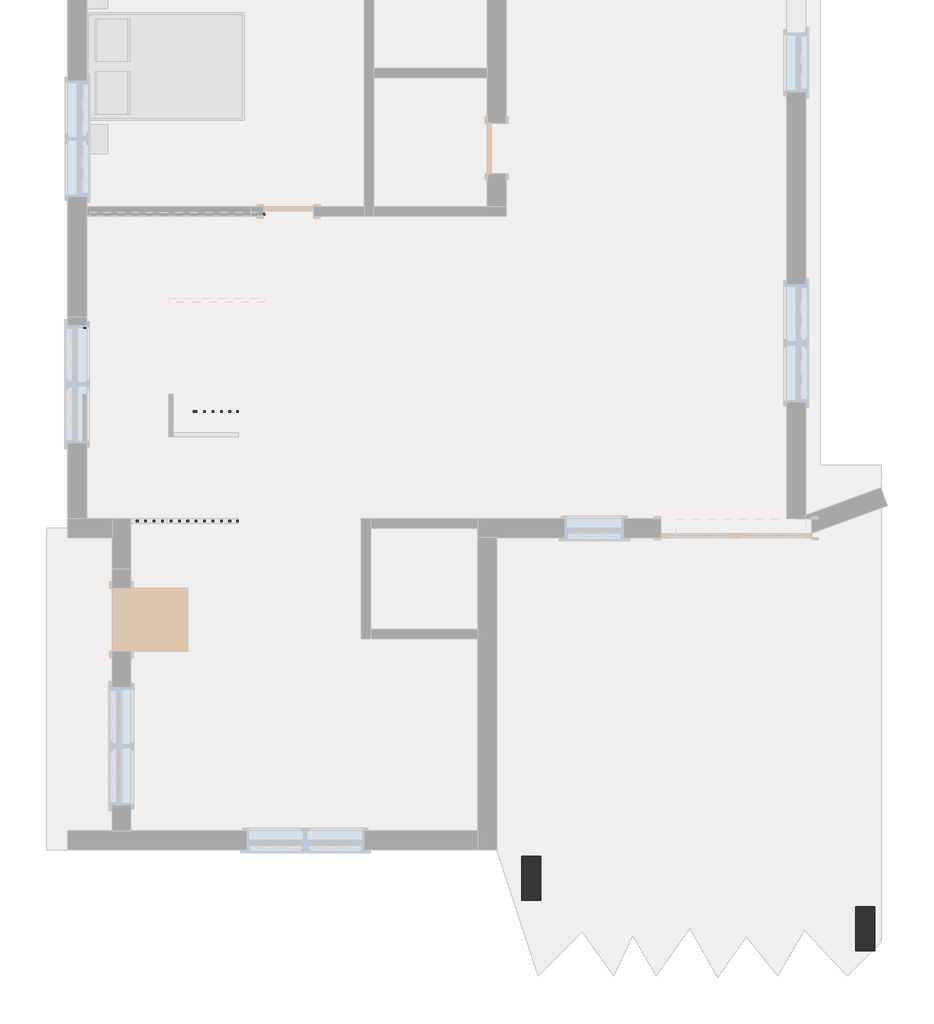
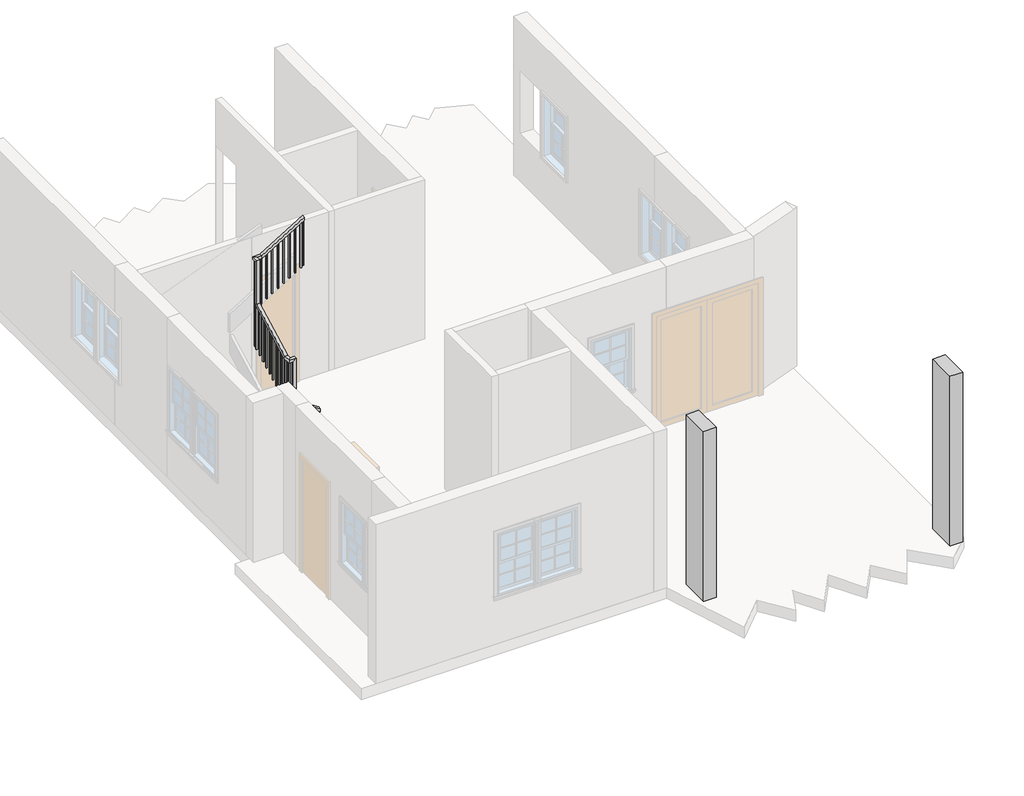
# One storey, part 2 of 3: 2 columns, 2 railings.
"""IFC4 building model written with IfcOpenShell, lengths in millimetres."""

from ifc_helpers import new_model, si_unit, frame, origin, place, context, project, spatial, polyline, outline, extrude, faceted_brep, transform, mapped, element, save
from components import column_b42c64cd

model = new_model("IFC4")

# Units and contexts
model_context = context("Model", 3, world=origin())
ifc_project = project(units=[si_unit("LENGTHUNIT", "METRE", prefix="MILLI")], contexts=[model_context])

# Site, building, storey
site = spatial("IfcSite", under=ifc_project)
building = spatial("IfcBuilding", under=site)
storey = spatial("IfcBuildingStorey", under=building, Elevation=3200.4)

# Columns
placement = place(None, origin())
column_shape = column_b42c64cd(model_context)
element("IfcColumn", 1, ObjectType="Rectangular Column : x9\"", at=placement, inside=storey, context=model_context, shape_type="MappedRepresentation", body=[
    mapped(column_shape, transform((-16875.4750314, 319.9223646, 0.0), x_axis=(1.0, 0.0, 0.0), y_axis=(0.0, 1.0, 0.0), z_axis=(0.0, 0.0, 1.0))),
])
element("IfcColumn", 2, ObjectType="Rectangular Column : x9\"", at=placement, inside=storey, context=model_context, shape_type="MappedRepresentation", body=[
    mapped(column_shape, transform((-12836.8750314, -289.6776354, 0.0), x_axis=(1.0, 0.0, 0.0), y_axis=(0.0, 1.0, 0.0), z_axis=(0.0, 0.0, 1.0))),
])

# Railings
element("IfcRailing", 3, ObjectType="Handrail - Rectangular", at=placement, inside=storey, context=model_context, shape_type="SolidModel", body=[
    faceted_brep([(-20418.7750314, 5933.3223646, 4470.4), (-20418.7750314, 5933.3223646, 4410.186276), (-20418.7750314, 5984.1223646, 4410.186276), (-20418.7750314, 5984.1223646, 4470.4), (-20850.5750314, 5933.3223646, 4745.1818182), (-20901.3750314, 5933.3223646, 4717.2953669), (-20901.3750314, 5984.1223646, 4717.2953669), (-20850.5750314, 5984.1223646, 4745.1818182), (-20850.5750314, 5933.3223646, 5574.9151515), (-20901.3750314, 5933.3223646, 5524.1151515), (-20901.3750314, 5984.1223646, 5524.1151515), (-20850.5750314, 5984.1223646, 5574.9151515), (-20977.5750314, 5933.3223646, 5574.9151515), (-20977.5750314, 5933.3223646, 5524.1151515), (-20926.7750314, 5984.1223646, 5524.1151515), (-20926.7750314, 5984.1223646, 5574.9151515), (-20977.5750314, 6060.3223646, 5574.9151515), (-20977.5750314, 6072.9586335, 5524.1151515), (-20926.7750314, 6072.9586335, 5524.1151515), (-20926.7750314, 6060.3223646, 5574.9151515), (-20977.5750314, 6923.9223646, 6032.8848485), (-20977.5750314, 6974.7223646, 6002.3231907), (-20926.7750314, 6974.7223646, 6002.3231907), (-20926.7750314, 6923.9223646, 6032.8848485), (-20088.5750314, 7050.9223646, 7315.2), (-20088.5750314, 7000.1223646, 7315.2), (-20088.5750314, 7000.1223646, 7255.7290495), (-20088.5750314, 7050.9223646, 7255.7290495), (-20836.3298984, 7050.9223646, 6800.573913), (-20850.5750314, 7050.9223646, 6851.373913), (-20836.3298984, 7000.1223646, 6800.573913), (-20850.5750314, 7000.1223646, 6851.373913), (-20977.5750314, 6923.9223646, 6851.373913), (-20977.5750314, 6974.7223646, 6800.573913), (-20926.7750314, 6974.7223646, 6800.573913), (-20926.7750314, 6923.9223646, 6851.373913), (-20977.5750314, 7050.9223646, 6851.373913), (-20977.5750314, 7050.9223646, 6800.573913), (-20926.7750314, 7000.1223646, 6800.573913), (-20926.7750314, 7000.1223646, 6851.373913)], [[[0, 1, 2, 3]], [[1, 0, 4, 5]], [[2, 1, 5, 6]], [[3, 2, 6, 7]], [[0, 3, 7, 4]], [[5, 4, 8, 9]], [[6, 5, 9, 10]], [[7, 6, 10, 11]], [[4, 7, 11, 8]], [[9, 8, 12, 13]], [[10, 9, 13, 14]], [[11, 10, 14, 15]], [[8, 11, 15, 12]], [[13, 12, 16, 17]], [[14, 13, 17, 18]], [[15, 14, 18, 19]], [[12, 15, 19, 16]], [[17, 16, 20, 21]], [[18, 17, 21, 22]], [[19, 18, 22, 23]], [[16, 19, 23, 20]], [[24, 25, 26, 27]], [[28, 29, 24, 27]], [[30, 28, 27, 26]], [[31, 30, 26, 25]], [[29, 31, 25, 24]], [[21, 20, 32, 33]], [[22, 21, 33, 34]], [[23, 22, 34, 35]], [[20, 23, 35, 32]], [[33, 32, 36, 37]], [[34, 33, 37, 38]], [[35, 34, 38, 39]], [[32, 35, 39, 36]], [[37, 36, 29, 28]], [[38, 37, 28, 30]], [[39, 38, 30, 31]], [[36, 39, 31, 29]]]),
    extrude(outline(polyline([(7230.6051365, -20129.8500314), (7219.0094843, -20148.9000314), (6369.8782609, -20148.9000314), (6369.8782609, -20129.8500314), (7230.6051365, -20129.8500314)])), frame((0.0, 7015.9973646, 0.0), z_axis=(0.0, 1.0, 0.0), x_axis=(0.0, 0.0, 1.0)), (0.0, 0.0, 1.0), 19.05),
    extrude(outline(polyline([(7168.7616582, -20231.4500314), (7157.166006, -20250.5000314), (6308.0347826, -20250.5000314), (6308.0347826, -20231.4500314), (7168.7616582, -20231.4500314)])), frame((0.0, 7015.9973646, 0.0), z_axis=(0.0, 1.0, 0.0), x_axis=(0.0, 0.0, 1.0)), (0.0, 0.0, 1.0), 19.05),
    extrude(outline(polyline([(7106.91818, -20333.0500314), (7095.3225278, -20352.1000314), (6246.1913043, -20352.1000314), (6246.1913043, -20333.0500314), (7106.91818, -20333.0500314)])), frame((0.0, 7015.9973646, 0.0), z_axis=(0.0, 1.0, 0.0), x_axis=(0.0, 0.0, 1.0)), (0.0, 0.0, 1.0), 19.05),
    extrude(outline(polyline([(7045.0747017, -20434.6500314), (7033.4790495, -20453.7000314), (6184.3478261, -20453.7000314), (6184.3478261, -20434.6500314), (7045.0747017, -20434.6500314)])), frame((0.0, 7015.9973646, 0.0), z_axis=(0.0, 1.0, 0.0), x_axis=(0.0, 0.0, 1.0)), (0.0, 0.0, 1.0), 19.05),
    extrude(outline(polyline([(6983.2312234, -20536.2500314), (6971.6355713, -20555.3000314), (6122.5043478, -20555.3000314), (6122.5043478, -20536.2500314), (6983.2312234, -20536.2500314)])), frame((0.0, 7015.9973646, 0.0), z_axis=(0.0, 1.0, 0.0), x_axis=(0.0, 0.0, 1.0)), (0.0, 0.0, 1.0), 19.05),
    extrude(outline(polyline([(6921.3877452, -20637.8500314), (6909.792093, -20656.9000314), (6060.6608696, -20656.9000314), (6060.6608696, -20637.8500314), (6921.3877452, -20637.8500314)])), frame((0.0, 7015.9973646, 0.0), z_axis=(0.0, 1.0, 0.0), x_axis=(0.0, 0.0, 1.0)), (0.0, 0.0, 1.0), 19.05),
    extrude(outline(polyline([(6859.5442669, -20739.4500314), (6847.9486147, -20758.5000314), (5998.8173913, -20758.5000314), (5998.8173913, -20739.4500314), (6859.5442669, -20739.4500314)])), frame((0.0, 7015.9973646, 0.0), z_axis=(0.0, 1.0, 0.0), x_axis=(0.0, 0.0, 1.0)), (0.0, 0.0, 1.0), 19.05),
    extrude(outline(polyline([(6797.7007887, -20841.0500314), (6786.1051365, -20860.1000314), (5936.973913, -20860.1000314), (5936.973913, -20841.0500314), (6797.7007887, -20841.0500314)])), frame((0.0, 7015.9973646, 0.0), z_axis=(0.0, 1.0, 0.0), x_axis=(0.0, 0.0, 1.0)), (0.0, 0.0, 1.0), 19.05),
    extrude(outline(polyline([(-20942.6500314, 6965.1973646), (-20961.7000314, 6965.1973646), (-20961.7000314, 6984.2473646), (-20942.6500314, 6984.2473646), (-20942.6500314, 6965.1973646)])), frame((0.0, 0.0, 5145.4242424), z_axis=(0.0, 0.0, 1.0), x_axis=(1.0, 0.0, 0.0)), (0.0, 0.0, 1.0), 1655.1496706),
    extrude(outline(polyline([(6863.5973646, 5943.3932665), (6882.6473646, 5953.4955392), (6882.6473646, 5091.5454545), (6863.5973646, 5091.5454545), (6863.5973646, 5943.3932665)])), frame((-20961.7000314, 0.0, 0.0), z_axis=(1.0, 0.0, 0.0), x_axis=(0.0, 1.0, 0.0)), (0.0, 0.0, 1.0), 19.05),
    extrude(outline(polyline([(6761.9973646, 5889.5144786), (6781.0473646, 5899.6167513), (6781.0473646, 5037.6666667), (6761.9973646, 5037.6666667), (6761.9973646, 5889.5144786)])), frame((-20961.7000314, 0.0, 0.0), z_axis=(1.0, 0.0, 0.0), x_axis=(0.0, 1.0, 0.0)), (0.0, 0.0, 1.0), 19.05),
    extrude(outline(polyline([(6660.3973646, 5835.6356907), (6679.4473646, 5845.7379635), (6679.4473646, 4983.7878788), (6660.3973646, 4983.7878788), (6660.3973646, 5835.6356907)])), frame((-20961.7000314, 0.0, 0.0), z_axis=(1.0, 0.0, 0.0), x_axis=(0.0, 1.0, 0.0)), (0.0, 0.0, 1.0), 19.05),
    extrude(outline(polyline([(6558.7973646, 5781.7569029), (6577.8473646, 5791.8591756), (6577.8473646, 4929.9090909), (6558.7973646, 4929.9090909), (6558.7973646, 5781.7569029)])), frame((-20961.7000314, 0.0, 0.0), z_axis=(1.0, 0.0, 0.0), x_axis=(0.0, 1.0, 0.0)), (0.0, 0.0, 1.0), 19.05),
    extrude(outline(polyline([(6457.1973646, 5727.878115), (6476.2473646, 5737.9803877), (6476.2473646, 4876.030303), (6457.1973646, 4876.030303), (6457.1973646, 5727.878115)])), frame((-20961.7000314, 0.0, 0.0), z_axis=(1.0, 0.0, 0.0), x_axis=(0.0, 1.0, 0.0)), (0.0, 0.0, 1.0), 19.05),
    extrude(outline(polyline([(6355.5973646, 5673.9993271), (6374.6473646, 5684.1015998), (6374.6473646, 4822.1515152), (6355.5973646, 4822.1515152), (6355.5973646, 5673.9993271)])), frame((-20961.7000314, 0.0, 0.0), z_axis=(1.0, 0.0, 0.0), x_axis=(0.0, 1.0, 0.0)), (0.0, 0.0, 1.0), 19.05),
    extrude(outline(polyline([(6253.9973646, 5620.1205392), (6273.0473646, 5630.2228119), (6273.0473646, 4768.2727273), (6253.9973646, 4768.2727273), (6253.9973646, 5620.1205392)])), frame((-20961.7000314, 0.0, 0.0), z_axis=(1.0, 0.0, 0.0), x_axis=(0.0, 1.0, 0.0)), (0.0, 0.0, 1.0), 19.05),
    extrude(outline(polyline([(6152.3973646, 5566.2417513), (6171.4473646, 5576.3440241), (6171.4473646, 4714.3939394), (6152.3973646, 4714.3939394), (6152.3973646, 5566.2417513)])), frame((-20961.7000314, 0.0, 0.0), z_axis=(1.0, 0.0, 0.0), x_axis=(0.0, 1.0, 0.0)), (0.0, 0.0, 1.0), 19.05),
    extrude(outline(polyline([(6050.7973646, 5512.3629635), (6069.8473646, 5522.4652362), (6069.8473646, 4660.5151515), (6050.7973646, 4660.5151515), (6050.7973646, 5512.3629635)])), frame((-20961.7000314, 0.0, 0.0), z_axis=(1.0, 0.0, 0.0), x_axis=(0.0, 1.0, 0.0)), (0.0, 0.0, 1.0), 19.05),
    extrude(outline(polyline([(-20917.2500314, 5968.2473646), (-20917.2500314, 5949.1973646), (-20936.3000314, 5949.1973646), (-20936.3000314, 5968.2473646), (-20917.2500314, 5968.2473646)])), frame((0.0, 0.0, 3879.2727273), z_axis=(0.0, 0.0, 1.0), x_axis=(1.0, 0.0, 0.0)), (0.0, 0.0, 1.0), 1644.8424242),
    extrude(outline(polyline([(4662.7430941, -20815.6500314), (4674.8658214, -20834.7000314), (3814.6181818, -20834.7000314), (3814.6181818, -20815.6500314), (4662.7430941, -20815.6500314)])), frame((0.0, 5949.1973646, 0.0), z_axis=(0.0, 1.0, 0.0), x_axis=(0.0, 0.0, 1.0)), (0.0, 0.0, 1.0), 19.05),
    extrude(outline(polyline([(4598.0885487, -20714.0500314), (4610.211276, -20733.1000314), (3749.9636364, -20733.1000314), (3749.9636364, -20714.0500314), (4598.0885487, -20714.0500314)])), frame((0.0, 5949.1973646, 0.0), z_axis=(0.0, 1.0, 0.0), x_axis=(0.0, 0.0, 1.0)), (0.0, 0.0, 1.0), 19.05),
    extrude(outline(polyline([(4533.4340032, -20612.4500314), (4545.5567305, -20631.5000314), (3685.3090909, -20631.5000314), (3685.3090909, -20612.4500314), (4533.4340032, -20612.4500314)])), frame((0.0, 5949.1973646, 0.0), z_axis=(0.0, 1.0, 0.0), x_axis=(0.0, 0.0, 1.0)), (0.0, 0.0, 1.0), 19.05),
    extrude(outline(polyline([(4468.7794578, -20510.8500314), (4480.9021851, -20529.9000314), (3620.6545455, -20529.9000314), (3620.6545455, -20510.8500314), (4468.7794578, -20510.8500314)])), frame((0.0, 5949.1973646, 0.0), z_axis=(0.0, 1.0, 0.0), x_axis=(0.0, 0.0, 1.0)), (0.0, 0.0, 1.0), 19.05),
    extrude(outline(polyline([(-20942.6500314, 7015.9973646), (-20961.7000314, 7015.9973646), (-20961.7000314, 7035.0473646), (-20942.6500314, 7035.0473646), (-20942.6500314, 7015.9973646)])), frame((0.0, 0.0, 5172.3636364), z_axis=(0.0, 0.0, 1.0), x_axis=(1.0, 0.0, 0.0)), (0.0, 0.0, 1.0), 1628.2102767),
    extrude(outline(polyline([(-20942.6500314, 5968.2473646), (-20942.6500314, 5949.1973646), (-20961.7000314, 5949.1973646), (-20961.7000314, 5968.2473646), (-20942.6500314, 5968.2473646)])), frame((0.0, 0.0, 3895.4363636), z_axis=(0.0, 0.0, 1.0), x_axis=(1.0, 0.0, 0.0)), (0.0, 0.0, 1.0), 1628.6787879),
    extrude(outline(polyline([(7255.7290495, -20088.5750314), (7244.1333973, -20107.6250314), (6395.0021739, -20107.6250314), (6395.0021739, -20088.5750314), (7255.7290495, -20088.5750314)])), frame((0.0, 7015.9973646, 0.0), z_axis=(0.0, 1.0, 0.0), x_axis=(0.0, 0.0, 1.0)), (0.0, 0.0, 1.0), 19.05),
    extrude(outline(polyline([(4410.186276, -20418.7750314), (4422.3090032, -20437.8250314), (3562.0613636, -20437.8250314), (3562.0613636, -20418.7750314), (4410.186276, -20418.7750314)])), frame((0.0, 5949.1973646, 0.0), z_axis=(0.0, 1.0, 0.0), x_axis=(0.0, 0.0, 1.0)), (0.0, 0.0, 1.0), 19.05),
])
element("IfcRailing", 4, ObjectType="Handrail - Rectangular", at=placement, inside=storey, context=model_context, shape_type="SolidModel", body=[
    faceted_brep([(-20418.7750314, 4612.5223646, 4470.4), (-20418.7750314, 4612.5223646, 4415.8938354), (-20418.7750314, 4663.3223646, 4415.8938354), (-20418.7750314, 4663.3223646, 4470.4), (-22171.3752061, 4612.5223646, 5151.9667346), (-22222.1752061, 4612.5223646, 5117.2161256), (-22222.1752061, 4663.3223646, 5117.2161256), (-22171.3752061, 4663.3223646, 5151.9667346), (-22171.3752061, 4612.5223646, 5181.600068), (-22222.1752061, 4612.5223646, 5130.800068), (-22222.1752061, 4663.3223646, 5130.800068), (-22171.3752061, 4663.3223646, 5181.600068), (-22298.3752061, 4612.5223646, 5181.600068), (-22298.3752061, 4612.5223646, 5130.800068), (-22247.5752061, 4663.3223646, 5130.800068), (-22247.5752061, 4663.3223646, 5181.600068), (-22298.3752061, 4739.5223646, 5181.600068), (-22298.3752061, 4739.5223646, 5130.800068), (-22247.5752061, 4739.5223646, 5130.800068), (-22247.5752061, 4739.5223646, 5181.600068), (-22298.3752061, 8371.7223646, 5181.600068), (-22298.3752061, 8371.7223646, 5130.800068), (-22247.5752061, 8320.9223646, 5130.800068), (-22247.5752061, 8320.9223646, 5181.600068), (-20088.5750314, 8371.7223646, 5181.600068), (-20088.5750314, 8320.9223646, 5181.600068), (-20088.5750314, 8320.9223646, 5130.800068), (-20088.5750314, 8371.7223646, 5130.800068)], [[[0, 1, 2, 3]], [[1, 0, 4, 5]], [[2, 1, 5, 6]], [[3, 2, 6, 7]], [[0, 3, 7, 4]], [[5, 4, 8, 9]], [[6, 5, 9, 10]], [[7, 6, 10, 11]], [[4, 7, 11, 8]], [[9, 8, 12, 13]], [[10, 9, 13, 14]], [[11, 10, 14, 15]], [[8, 11, 15, 12]], [[13, 12, 16, 17]], [[14, 13, 17, 18]], [[15, 14, 18, 19]], [[12, 15, 19, 16]], [[17, 16, 20, 21]], [[18, 17, 21, 22]], [[19, 18, 22, 23]], [[16, 19, 23, 20]], [[24, 25, 26, 27]], [[21, 20, 24, 27]], [[22, 21, 27, 26]], [[23, 22, 26, 25]], [[20, 23, 25, 24]]]),
    extrude(outline(polyline([(-20148.9002061, 8355.8473646), (-20129.8502061, 8355.8473646), (-20129.8502061, 8336.7973646), (-20148.9002061, 8336.7973646), (-20148.9002061, 8355.8473646)])), frame((0.0, 0.0, 4267.200068), z_axis=(0.0, 0.0, 1.0), x_axis=(1.0, 0.0, 0.0)), (0.0, 0.0, 1.0), 863.6),
    extrude(outline(polyline([(-20250.5002061, 8355.8473646), (-20231.4502061, 8355.8473646), (-20231.4502061, 8336.7973646), (-20250.5002061, 8336.7973646), (-20250.5002061, 8355.8473646)])), frame((0.0, 0.0, 4267.200068), z_axis=(0.0, 0.0, 1.0), x_axis=(1.0, 0.0, 0.0)), (0.0, 0.0, 1.0), 863.6),
    extrude(outline(polyline([(-20352.1002061, 8355.8473646), (-20333.0502061, 8355.8473646), (-20333.0502061, 8336.7973646), (-20352.1002061, 8336.7973646), (-20352.1002061, 8355.8473646)])), frame((0.0, 0.0, 4267.200068), z_axis=(0.0, 0.0, 1.0), x_axis=(1.0, 0.0, 0.0)), (0.0, 0.0, 1.0), 863.6),
    extrude(outline(polyline([(-20453.7002061, 8355.8473646), (-20434.6502061, 8355.8473646), (-20434.6502061, 8336.7973646), (-20453.7002061, 8336.7973646), (-20453.7002061, 8355.8473646)])), frame((0.0, 0.0, 4267.200068), z_axis=(0.0, 0.0, 1.0), x_axis=(1.0, 0.0, 0.0)), (0.0, 0.0, 1.0), 863.6),
    extrude(outline(polyline([(-20555.3002061, 8355.8473646), (-20536.2502061, 8355.8473646), (-20536.2502061, 8336.7973646), (-20555.3002061, 8336.7973646), (-20555.3002061, 8355.8473646)])), frame((0.0, 0.0, 4267.200068), z_axis=(0.0, 0.0, 1.0), x_axis=(1.0, 0.0, 0.0)), (0.0, 0.0, 1.0), 863.6),
    extrude(outline(polyline([(-20656.9002061, 8355.8473646), (-20637.8502061, 8355.8473646), (-20637.8502061, 8336.7973646), (-20656.9002061, 8336.7973646), (-20656.9002061, 8355.8473646)])), frame((0.0, 0.0, 4267.200068), z_axis=(0.0, 0.0, 1.0), x_axis=(1.0, 0.0, 0.0)), (0.0, 0.0, 1.0), 863.6),
    extrude(outline(polyline([(-20758.5002061, 8355.8473646), (-20739.4502061, 8355.8473646), (-20739.4502061, 8336.7973646), (-20758.5002061, 8336.7973646), (-20758.5002061, 8355.8473646)])), frame((0.0, 0.0, 4267.200068), z_axis=(0.0, 0.0, 1.0), x_axis=(1.0, 0.0, 0.0)), (0.0, 0.0, 1.0), 863.6),
    extrude(outline(polyline([(-20860.1002061, 8355.8473646), (-20841.0502061, 8355.8473646), (-20841.0502061, 8336.7973646), (-20860.1002061, 8336.7973646), (-20860.1002061, 8355.8473646)])), frame((0.0, 0.0, 4267.200068), z_axis=(0.0, 0.0, 1.0), x_axis=(1.0, 0.0, 0.0)), (0.0, 0.0, 1.0), 863.6),
    extrude(outline(polyline([(-20961.7002061, 8355.8473646), (-20942.6502061, 8355.8473646), (-20942.6502061, 8336.7973646), (-20961.7002061, 8336.7973646), (-20961.7002061, 8355.8473646)])), frame((0.0, 0.0, 4267.200068), z_axis=(0.0, 0.0, 1.0), x_axis=(1.0, 0.0, 0.0)), (0.0, 0.0, 1.0), 863.6),
    extrude(outline(polyline([(-21063.3002061, 8355.8473646), (-21044.2502061, 8355.8473646), (-21044.2502061, 8336.7973646), (-21063.3002061, 8336.7973646), (-21063.3002061, 8355.8473646)])), frame((0.0, 0.0, 4267.200068), z_axis=(0.0, 0.0, 1.0), x_axis=(1.0, 0.0, 0.0)), (0.0, 0.0, 1.0), 863.6),
    extrude(outline(polyline([(-21164.9002061, 8355.8473646), (-21145.8502061, 8355.8473646), (-21145.8502061, 8336.7973646), (-21164.9002061, 8336.7973646), (-21164.9002061, 8355.8473646)])), frame((0.0, 0.0, 4267.200068), z_axis=(0.0, 0.0, 1.0), x_axis=(1.0, 0.0, 0.0)), (0.0, 0.0, 1.0), 863.6),
    extrude(outline(polyline([(-21266.5002061, 8355.8473646), (-21247.4502061, 8355.8473646), (-21247.4502061, 8336.7973646), (-21266.5002061, 8336.7973646), (-21266.5002061, 8355.8473646)])), frame((0.0, 0.0, 4267.200068), z_axis=(0.0, 0.0, 1.0), x_axis=(1.0, 0.0, 0.0)), (0.0, 0.0, 1.0), 863.6),
    extrude(outline(polyline([(-21368.1002061, 8355.8473646), (-21349.0502061, 8355.8473646), (-21349.0502061, 8336.7973646), (-21368.1002061, 8336.7973646), (-21368.1002061, 8355.8473646)])), frame((0.0, 0.0, 4267.200068), z_axis=(0.0, 0.0, 1.0), x_axis=(1.0, 0.0, 0.0)), (0.0, 0.0, 1.0), 863.6),
    extrude(outline(polyline([(-21469.7002061, 8355.8473646), (-21450.6502061, 8355.8473646), (-21450.6502061, 8336.7973646), (-21469.7002061, 8336.7973646), (-21469.7002061, 8355.8473646)])), frame((0.0, 0.0, 4267.200068), z_axis=(0.0, 0.0, 1.0), x_axis=(1.0, 0.0, 0.0)), (0.0, 0.0, 1.0), 863.6),
    extrude(outline(polyline([(-21571.3002061, 8355.8473646), (-21552.2502061, 8355.8473646), (-21552.2502061, 8336.7973646), (-21571.3002061, 8336.7973646), (-21571.3002061, 8355.8473646)])), frame((0.0, 0.0, 4267.200068), z_axis=(0.0, 0.0, 1.0), x_axis=(1.0, 0.0, 0.0)), (0.0, 0.0, 1.0), 863.6),
    extrude(outline(polyline([(-21672.9002061, 8355.8473646), (-21653.8502061, 8355.8473646), (-21653.8502061, 8336.7973646), (-21672.9002061, 8336.7973646), (-21672.9002061, 8355.8473646)])), frame((0.0, 0.0, 4267.200068), z_axis=(0.0, 0.0, 1.0), x_axis=(1.0, 0.0, 0.0)), (0.0, 0.0, 1.0), 863.6),
    extrude(outline(polyline([(-21774.5002061, 8355.8473646), (-21755.4502061, 8355.8473646), (-21755.4502061, 8336.7973646), (-21774.5002061, 8336.7973646), (-21774.5002061, 8355.8473646)])), frame((0.0, 0.0, 4267.200068), z_axis=(0.0, 0.0, 1.0), x_axis=(1.0, 0.0, 0.0)), (0.0, 0.0, 1.0), 863.6),
    extrude(outline(polyline([(-21876.1002061, 8355.8473646), (-21857.0502061, 8355.8473646), (-21857.0502061, 8336.7973646), (-21876.1002061, 8336.7973646), (-21876.1002061, 8355.8473646)])), frame((0.0, 0.0, 4267.200068), z_axis=(0.0, 0.0, 1.0), x_axis=(1.0, 0.0, 0.0)), (0.0, 0.0, 1.0), 863.6),
    extrude(outline(polyline([(-21977.7002061, 8355.8473646), (-21958.6502061, 8355.8473646), (-21958.6502061, 8336.7973646), (-21977.7002061, 8336.7973646), (-21977.7002061, 8355.8473646)])), frame((0.0, 0.0, 4267.200068), z_axis=(0.0, 0.0, 1.0), x_axis=(1.0, 0.0, 0.0)), (0.0, 0.0, 1.0), 863.6),
    extrude(outline(polyline([(-22079.3002061, 8355.8473646), (-22060.2502061, 8355.8473646), (-22060.2502061, 8336.7973646), (-22079.3002061, 8336.7973646), (-22079.3002061, 8355.8473646)])), frame((0.0, 0.0, 4267.200068), z_axis=(0.0, 0.0, 1.0), x_axis=(1.0, 0.0, 0.0)), (0.0, 0.0, 1.0), 863.6),
    extrude(outline(polyline([(-22180.9002061, 8355.8473646), (-22161.8502061, 8355.8473646), (-22161.8502061, 8336.7973646), (-22180.9002061, 8336.7973646), (-22180.9002061, 8355.8473646)])), frame((0.0, 0.0, 4267.200068), z_axis=(0.0, 0.0, 1.0), x_axis=(1.0, 0.0, 0.0)), (0.0, 0.0, 1.0), 863.6),
    extrude(outline(polyline([(-22282.5002061, 8285.9973646), (-22282.5002061, 8305.0473646), (-22263.4502061, 8305.0473646), (-22263.4502061, 8285.9973646), (-22282.5002061, 8285.9973646)])), frame((0.0, 0.0, 4267.200068), z_axis=(0.0, 0.0, 1.0), x_axis=(1.0, 0.0, 0.0)), (0.0, 0.0, 1.0), 863.6),
    extrude(outline(polyline([(-22282.5002061, 8184.3973646), (-22282.5002061, 8203.4473646), (-22263.4502061, 8203.4473646), (-22263.4502061, 8184.3973646), (-22282.5002061, 8184.3973646)])), frame((0.0, 0.0, 4267.200068), z_axis=(0.0, 0.0, 1.0), x_axis=(1.0, 0.0, 0.0)), (0.0, 0.0, 1.0), 863.6),
    extrude(outline(polyline([(-22282.5002061, 8082.7973646), (-22282.5002061, 8101.8473646), (-22263.4502061, 8101.8473646), (-22263.4502061, 8082.7973646), (-22282.5002061, 8082.7973646)])), frame((0.0, 0.0, 4267.200068), z_axis=(0.0, 0.0, 1.0), x_axis=(1.0, 0.0, 0.0)), (0.0, 0.0, 1.0), 863.6),
    extrude(outline(polyline([(-22282.5002061, 7981.1973646), (-22282.5002061, 8000.2473646), (-22263.4502061, 8000.2473646), (-22263.4502061, 7981.1973646), (-22282.5002061, 7981.1973646)])), frame((0.0, 0.0, 4267.200068), z_axis=(0.0, 0.0, 1.0), x_axis=(1.0, 0.0, 0.0)), (0.0, 0.0, 1.0), 863.6),
    extrude(outline(polyline([(-22282.5002061, 7879.5973646), (-22282.5002061, 7898.6473646), (-22263.4502061, 7898.6473646), (-22263.4502061, 7879.5973646), (-22282.5002061, 7879.5973646)])), frame((0.0, 0.0, 4267.200068), z_axis=(0.0, 0.0, 1.0), x_axis=(1.0, 0.0, 0.0)), (0.0, 0.0, 1.0), 863.6),
    extrude(outline(polyline([(-22282.5002061, 7777.9973646), (-22282.5002061, 7797.0473646), (-22263.4502061, 7797.0473646), (-22263.4502061, 7777.9973646), (-22282.5002061, 7777.9973646)])), frame((0.0, 0.0, 4267.200068), z_axis=(0.0, 0.0, 1.0), x_axis=(1.0, 0.0, 0.0)), (0.0, 0.0, 1.0), 863.6),
    extrude(outline(polyline([(-22282.5002061, 7676.3973646), (-22282.5002061, 7695.4473646), (-22263.4502061, 7695.4473646), (-22263.4502061, 7676.3973646), (-22282.5002061, 7676.3973646)])), frame((0.0, 0.0, 4267.200068), z_axis=(0.0, 0.0, 1.0), x_axis=(1.0, 0.0, 0.0)), (0.0, 0.0, 1.0), 863.6),
    extrude(outline(polyline([(-22282.5002061, 7574.7973646), (-22282.5002061, 7593.8473646), (-22263.4502061, 7593.8473646), (-22263.4502061, 7574.7973646), (-22282.5002061, 7574.7973646)])), frame((0.0, 0.0, 4267.200068), z_axis=(0.0, 0.0, 1.0), x_axis=(1.0, 0.0, 0.0)), (0.0, 0.0, 1.0), 863.6),
    extrude(outline(polyline([(-22282.5002061, 7473.1973646), (-22282.5002061, 7492.2473646), (-22263.4502061, 7492.2473646), (-22263.4502061, 7473.1973646), (-22282.5002061, 7473.1973646)])), frame((0.0, 0.0, 4267.200068), z_axis=(0.0, 0.0, 1.0), x_axis=(1.0, 0.0, 0.0)), (0.0, 0.0, 1.0), 863.6),
    extrude(outline(polyline([(-22282.5002061, 7371.5973646), (-22282.5002061, 7390.6473646), (-22263.4502061, 7390.6473646), (-22263.4502061, 7371.5973646), (-22282.5002061, 7371.5973646)])), frame((0.0, 0.0, 4267.200068), z_axis=(0.0, 0.0, 1.0), x_axis=(1.0, 0.0, 0.0)), (0.0, 0.0, 1.0), 863.6),
    extrude(outline(polyline([(-22282.5002061, 7269.9973646), (-22282.5002061, 7289.0473646), (-22263.4502061, 7289.0473646), (-22263.4502061, 7269.9973646), (-22282.5002061, 7269.9973646)])), frame((0.0, 0.0, 4267.200068), z_axis=(0.0, 0.0, 1.0), x_axis=(1.0, 0.0, 0.0)), (0.0, 0.0, 1.0), 863.6),
    extrude(outline(polyline([(-22282.5002061, 7168.3973646), (-22282.5002061, 7187.4473646), (-22263.4502061, 7187.4473646), (-22263.4502061, 7168.3973646), (-22282.5002061, 7168.3973646)])), frame((0.0, 0.0, 4267.200068), z_axis=(0.0, 0.0, 1.0), x_axis=(1.0, 0.0, 0.0)), (0.0, 0.0, 1.0), 863.6),
    extrude(outline(polyline([(-22282.5002061, 7066.7973646), (-22282.5002061, 7085.8473646), (-22263.4502061, 7085.8473646), (-22263.4502061, 7066.7973646), (-22282.5002061, 7066.7973646)])), frame((0.0, 0.0, 4267.200068), z_axis=(0.0, 0.0, 1.0), x_axis=(1.0, 0.0, 0.0)), (0.0, 0.0, 1.0), 863.6),
    extrude(outline(polyline([(-22282.5002061, 6965.1973646), (-22282.5002061, 6984.2473646), (-22263.4502061, 6984.2473646), (-22263.4502061, 6965.1973646), (-22282.5002061, 6965.1973646)])), frame((0.0, 0.0, 4267.200068), z_axis=(0.0, 0.0, 1.0), x_axis=(1.0, 0.0, 0.0)), (0.0, 0.0, 1.0), 863.6),
    extrude(outline(polyline([(6882.6473646, 5130.800068), (6882.6473646, 5124.2894652), (6863.5973646, 5114.1871925), (6863.5973646, 5130.800068), (6882.6473646, 5130.800068)])), frame((-22282.5002061, 0.0, 0.0), z_axis=(1.0, 0.0, 0.0), x_axis=(0.0, 1.0, 0.0)), (0.0, 0.0, 1.0), 19.05),
    extrude(outline(polyline([(6781.0473646, 5130.800068), (6781.0473646, 5070.4106774), (6761.9973646, 5060.3084046), (6761.9973646, 5130.800068), (6781.0473646, 5130.800068)])), frame((-22282.5002061, 0.0, 0.0), z_axis=(1.0, 0.0, 0.0), x_axis=(0.0, 1.0, 0.0)), (0.0, 0.0, 1.0), 19.05),
    extrude(outline(polyline([(6679.4473646, 5130.800068), (6679.4473646, 5016.5318895), (6660.3973646, 5006.4296168), (6660.3973646, 5130.800068), (6679.4473646, 5130.800068)])), frame((-22282.5002061, 0.0, 0.0), z_axis=(1.0, 0.0, 0.0), x_axis=(0.0, 1.0, 0.0)), (0.0, 0.0, 1.0), 19.05),
    extrude(outline(polyline([(6577.8473646, 5130.800068), (6577.8473646, 4962.6531016), (6558.7973646, 4952.5508289), (6558.7973646, 5130.800068), (6577.8473646, 5130.800068)])), frame((-22282.5002061, 0.0, 0.0), z_axis=(1.0, 0.0, 0.0), x_axis=(0.0, 1.0, 0.0)), (0.0, 0.0, 1.0), 19.05),
    extrude(outline(polyline([(6476.2473646, 5130.800068), (6476.2473646, 4908.7743137), (6457.1973646, 4898.672041), (6457.1973646, 5130.800068), (6476.2473646, 5130.800068)])), frame((-22282.5002061, 0.0, 0.0), z_axis=(1.0, 0.0, 0.0), x_axis=(0.0, 1.0, 0.0)), (0.0, 0.0, 1.0), 19.05),
    extrude(outline(polyline([(6374.6473646, 5130.800068), (6374.6473646, 4854.8955258), (6355.5973646, 4844.7932531), (6355.5973646, 5130.800068), (6374.6473646, 5130.800068)])), frame((-22282.5002061, 0.0, 0.0), z_axis=(1.0, 0.0, 0.0), x_axis=(0.0, 1.0, 0.0)), (0.0, 0.0, 1.0), 19.05),
    extrude(outline(polyline([(6273.0473646, 5130.800068), (6273.0473646, 4801.016738), (6253.9973646, 4790.9144652), (6253.9973646, 5130.800068), (6273.0473646, 5130.800068)])), frame((-22282.5002061, 0.0, 0.0), z_axis=(1.0, 0.0, 0.0), x_axis=(0.0, 1.0, 0.0)), (0.0, 0.0, 1.0), 19.05),
    extrude(outline(polyline([(6171.4473646, 5130.800068), (6171.4473646, 4747.1379501), (6152.3973646, 4737.0356774), (6152.3973646, 5130.800068), (6171.4473646, 5130.800068)])), frame((-22282.5002061, 0.0, 0.0), z_axis=(1.0, 0.0, 0.0), x_axis=(0.0, 1.0, 0.0)), (0.0, 0.0, 1.0), 19.05),
    extrude(outline(polyline([(6069.8473646, 5130.800068), (6069.8473646, 4693.2591622), (6050.7973646, 4683.1568895), (6050.7973646, 5130.800068), (6069.8473646, 5130.800068)])), frame((-22282.5002061, 0.0, 0.0), z_axis=(1.0, 0.0, 0.0), x_axis=(0.0, 1.0, 0.0)), (0.0, 0.0, 1.0), 19.05),
    extrude(outline(polyline([(5968.2473646, 5130.800068), (5968.2473646, 4639.3803743), (5949.1973646, 4629.2781016), (5949.1973646, 5130.800068), (5968.2473646, 5130.800068)])), frame((-22282.5002061, 0.0, 0.0), z_axis=(1.0, 0.0, 0.0), x_axis=(0.0, 1.0, 0.0)), (0.0, 0.0, 1.0), 19.05),
    extrude(outline(polyline([(5866.6473646, 5130.800068), (5866.6473646, 4585.5015865), (5847.5973646, 4575.3993137), (5847.5973646, 5130.800068), (5866.6473646, 5130.800068)])), frame((-22282.5002061, 0.0, 0.0), z_axis=(1.0, 0.0, 0.0), x_axis=(0.0, 1.0, 0.0)), (0.0, 0.0, 1.0), 19.05),
    extrude(outline(polyline([(5765.0473646, 5130.800068), (5765.0473646, 4531.6227986), (5745.9973646, 4521.5205258), (5745.9973646, 5130.800068), (5765.0473646, 5130.800068)])), frame((-22282.5002061, 0.0, 0.0), z_axis=(1.0, 0.0, 0.0), x_axis=(0.0, 1.0, 0.0)), (0.0, 0.0, 1.0), 19.05),
    extrude(outline(polyline([(5663.4473646, 5130.800068), (5663.4473646, 4477.7440107), (5644.3973646, 4467.641738), (5644.3973646, 5130.800068), (5663.4473646, 5130.800068)])), frame((-22282.5002061, 0.0, 0.0), z_axis=(1.0, 0.0, 0.0), x_axis=(0.0, 1.0, 0.0)), (0.0, 0.0, 1.0), 19.05),
    extrude(outline(polyline([(5561.8473646, 5130.800068), (5561.8473646, 4423.8652228), (5542.7973646, 4413.7629501), (5542.7973646, 5130.800068), (5561.8473646, 5130.800068)])), frame((-22282.5002061, 0.0, 0.0), z_axis=(1.0, 0.0, 0.0), x_axis=(0.0, 1.0, 0.0)), (0.0, 0.0, 1.0), 19.05),
    extrude(outline(polyline([(5460.2473646, 5130.800068), (5460.2473646, 4369.9864349), (5441.1973646, 4359.8841622), (5441.1973646, 5130.800068), (5460.2473646, 5130.800068)])), frame((-22282.5002061, 0.0, 0.0), z_axis=(1.0, 0.0, 0.0), x_axis=(0.0, 1.0, 0.0)), (0.0, 0.0, 1.0), 19.05),
    extrude(outline(polyline([(5358.6473646, 5130.800068), (5358.6473646, 4316.1076471), (5339.5973646, 4306.0053743), (5339.5973646, 5130.800068), (5358.6473646, 5130.800068)])), frame((-22282.5002061, 0.0, 0.0), z_axis=(1.0, 0.0, 0.0), x_axis=(0.0, 1.0, 0.0)), (0.0, 0.0, 1.0), 19.05),
    extrude(outline(polyline([(5257.0473646, 5130.800068), (5257.0473646, 4262.2288592), (5237.9973646, 4252.1265865), (5237.9973646, 5130.800068), (5257.0473646, 5130.800068)])), frame((-22282.5002061, 0.0, 0.0), z_axis=(1.0, 0.0, 0.0), x_axis=(0.0, 1.0, 0.0)), (0.0, 0.0, 1.0), 19.05),
    extrude(outline(polyline([(5155.4473646, 5130.800068), (5155.4473646, 4208.3500713), (5136.3973646, 4198.2477986), (5136.3973646, 5130.800068), (5155.4473646, 5130.800068)])), frame((-22282.5002061, 0.0, 0.0), z_axis=(1.0, 0.0, 0.0), x_axis=(0.0, 1.0, 0.0)), (0.0, 0.0, 1.0), 19.05),
    extrude(outline(polyline([(5053.8473646, 5130.800068), (5053.8473646, 4154.4712834), (5034.7973646, 4144.3690107), (5034.7973646, 5130.800068), (5053.8473646, 5130.800068)])), frame((-22282.5002061, 0.0, 0.0), z_axis=(1.0, 0.0, 0.0), x_axis=(0.0, 1.0, 0.0)), (0.0, 0.0, 1.0), 19.05),
    extrude(outline(polyline([(4952.2473646, 5130.800068), (4952.2473646, 4100.5924955), (4933.1973646, 4090.4902228), (4933.1973646, 5130.800068), (4952.2473646, 5130.800068)])), frame((-22282.5002061, 0.0, 0.0), z_axis=(1.0, 0.0, 0.0), x_axis=(0.0, 1.0, 0.0)), (0.0, 0.0, 1.0), 19.05),
    extrude(outline(polyline([(-22282.5002061, 4831.5973646), (-22282.5002061, 4850.6473646), (-22263.4502061, 4850.6473646), (-22263.4502061, 4831.5973646), (-22282.5002061, 4831.5973646)])), frame((0.0, 0.0, 4267.200068), z_axis=(0.0, 0.0, 1.0), x_axis=(1.0, 0.0, 0.0)), (0.0, 0.0, 1.0), 863.6),
    extrude(outline(polyline([(-22282.5002061, 4729.9973646), (-22282.5002061, 4749.0473646), (-22263.4502061, 4749.0473646), (-22263.4502061, 4729.9973646), (-22282.5002061, 4729.9973646)])), frame((0.0, 0.0, 4267.200068), z_axis=(0.0, 0.0, 1.0), x_axis=(1.0, 0.0, 0.0)), (0.0, 0.0, 1.0), 863.6),
    extrude(outline(polyline([(-22238.0500314, 4628.3973646), (-22257.1000314, 4628.3973646), (-22257.1000314, 4647.4473646), (-22238.0500314, 4647.4473646), (-22238.0500314, 4628.3973646)])), frame((0.0, 0.0, 4267.2), z_axis=(0.0, 0.0, 1.0), x_axis=(1.0, 0.0, 0.0)), (0.0, 0.0, 1.0), 863.600068),
    extrude(outline(polyline([(5091.286891, -22155.5000314), (4227.6888889, -22155.5000314), (4227.6888889, -22136.4500314), (5083.8785577, -22136.4500314), (5091.286891, -22155.5000314)])), frame((0.0, 4628.3973646, 0.0), z_axis=(0.0, 1.0, 0.0), x_axis=(0.0, 0.0, 1.0)), (0.0, 0.0, 1.0), 19.05),
    extrude(outline(polyline([(5051.7757799, -22053.9000314), (4188.1777778, -22053.9000314), (4188.1777778, -22034.8500314), (5044.3674465, -22034.8500314), (5051.7757799, -22053.9000314)])), frame((0.0, 4628.3973646, 0.0), z_axis=(0.0, 1.0, 0.0), x_axis=(0.0, 0.0, 1.0)), (0.0, 0.0, 1.0), 19.05),
    extrude(outline(polyline([(5012.2646688, -21952.3000314), (4148.6666667, -21952.3000314), (4148.6666667, -21933.2500314), (5004.8563354, -21933.2500314), (5012.2646688, -21952.3000314)])), frame((0.0, 4628.3973646, 0.0), z_axis=(0.0, 1.0, 0.0), x_axis=(0.0, 0.0, 1.0)), (0.0, 0.0, 1.0), 19.05),
    extrude(outline(polyline([(4972.7535577, -21850.7000314), (3947.3746925, -21850.7000314), (3947.3746925, -21831.6500314), (4965.3452243, -21831.6500314), (4972.7535577, -21850.7000314)])), frame((0.0, 4628.3973646, 0.0), z_axis=(0.0, 1.0, 0.0), x_axis=(0.0, 0.0, 1.0)), (0.0, 0.0, 1.0), 19.05),
    extrude(outline(polyline([(4933.2424465, -21749.1000314), (3947.3746925, -21749.1000314), (3947.3746925, -21730.0500314), (4925.8341132, -21730.0500314), (4933.2424465, -21749.1000314)])), frame((0.0, 4628.3973646, 0.0), z_axis=(0.0, 1.0, 0.0), x_axis=(0.0, 0.0, 1.0)), (0.0, 0.0, 1.0), 19.05),
    extrude(outline(polyline([(4893.7313354, -21647.5000314), (3947.3746925, -21647.5000314), (3947.3746925, -21628.4500314), (4886.3230021, -21628.4500314), (4893.7313354, -21647.5000314)])), frame((0.0, 4628.3973646, 0.0), z_axis=(0.0, 1.0, 0.0), x_axis=(0.0, 0.0, 1.0)), (0.0, 0.0, 1.0), 19.05),
    extrude(outline(polyline([(4854.2202243, -21545.9000314), (3947.3746925, -21545.9000314), (3947.3746925, -21526.8500314), (4846.811891, -21526.8500314), (4854.2202243, -21545.9000314)])), frame((0.0, 4628.3973646, 0.0), z_axis=(0.0, 1.0, 0.0), x_axis=(0.0, 0.0, 1.0)), (0.0, 0.0, 1.0), 19.05),
    extrude(outline(polyline([(4814.7091132, -21444.3000314), (3947.3746925, -21444.3000314), (3947.3746925, -21425.2500314), (4807.3007799, -21425.2500314), (4814.7091132, -21444.3000314)])), frame((0.0, 4628.3973646, 0.0), z_axis=(0.0, 1.0, 0.0), x_axis=(0.0, 0.0, 1.0)), (0.0, 0.0, 1.0), 19.05),
    extrude(outline(polyline([(4775.1980021, -21342.7000314), (3947.3746925, -21342.7000314), (3947.3746925, -21323.6500314), (4767.7896688, -21323.6500314), (4775.1980021, -21342.7000314)])), frame((0.0, 4628.3973646, 0.0), z_axis=(0.0, 1.0, 0.0), x_axis=(0.0, 0.0, 1.0)), (0.0, 0.0, 1.0), 19.05),
    extrude(outline(polyline([(4735.686891, -21241.1000314), (3936.3770181, -21241.1000314), (3929.8188214, -21222.0500314), (4728.2785577, -21222.0500314), (4735.686891, -21241.1000314)])), frame((0.0, 4628.3973646, 0.0), z_axis=(0.0, 1.0, 0.0), x_axis=(0.0, 0.0, 1.0)), (0.0, 0.0, 1.0), 19.05),
    extrude(outline(polyline([(4696.1757799, -21139.5000314), (3901.3999689, -21139.5000314), (3894.8417722, -21120.4500314), (4688.7674465, -21120.4500314), (4696.1757799, -21139.5000314)])), frame((0.0, 4628.3973646, 0.0), z_axis=(0.0, 1.0, 0.0), x_axis=(0.0, 0.0, 1.0)), (0.0, 0.0, 1.0), 19.05),
    extrude(outline(polyline([(4656.6646688, -21037.9000314), (3866.4229198, -21037.9000314), (3859.864723, -21018.8500314), (4649.2563354, -21018.8500314), (4656.6646688, -21037.9000314)])), frame((0.0, 4628.3973646, 0.0), z_axis=(0.0, 1.0, 0.0), x_axis=(0.0, 0.0, 1.0)), (0.0, 0.0, 1.0), 19.05),
    extrude(outline(polyline([(4617.1535577, -20936.3000314), (3831.4458706, -20936.3000314), (3824.8876739, -20917.2500314), (4609.7452243, -20917.2500314), (4617.1535577, -20936.3000314)])), frame((0.0, 4628.3973646, 0.0), z_axis=(0.0, 1.0, 0.0), x_axis=(0.0, 0.0, 1.0)), (0.0, 0.0, 1.0), 19.05),
    extrude(outline(polyline([(4577.6424465, -20834.7000314), (3796.4688214, -20834.7000314), (3789.9106247, -20815.6500314), (4570.2341132, -20815.6500314), (4577.6424465, -20834.7000314)])), frame((0.0, 4628.3973646, 0.0), z_axis=(0.0, 1.0, 0.0), x_axis=(0.0, 0.0, 1.0)), (0.0, 0.0, 1.0), 19.05),
    extrude(outline(polyline([(4538.1313354, -20733.1000314), (3761.4917722, -20733.1000314), (3754.9335755, -20714.0500314), (4530.7230021, -20714.0500314), (4538.1313354, -20733.1000314)])), frame((0.0, 4628.3973646, 0.0), z_axis=(0.0, 1.0, 0.0), x_axis=(0.0, 0.0, 1.0)), (0.0, 0.0, 1.0), 19.05),
    extrude(outline(polyline([(4498.6202243, -20631.5000314), (3726.514723, -20631.5000314), (3719.9565263, -20612.4500314), (4491.211891, -20612.4500314), (4498.6202243, -20631.5000314)])), frame((0.0, 4628.3973646, 0.0), z_axis=(0.0, 1.0, 0.0), x_axis=(0.0, 0.0, 1.0)), (0.0, 0.0, 1.0), 19.05),
    extrude(outline(polyline([(4459.1091132, -20529.9000314), (3691.5376739, -20529.9000314), (3684.9794771, -20510.8500314), (4451.7007799, -20510.8500314), (4459.1091132, -20529.9000314)])), frame((0.0, 4628.3973646, 0.0), z_axis=(0.0, 1.0, 0.0), x_axis=(0.0, 0.0, 1.0)), (0.0, 0.0, 1.0), 19.05),
    extrude(outline(polyline([(-22282.5002061, 8336.7973646), (-22282.5002061, 8355.8473646), (-22263.4502061, 8355.8473646), (-22263.4502061, 8336.7973646), (-22282.5002061, 8336.7973646)])), frame((0.0, 0.0, 4267.200068), z_axis=(0.0, 0.0, 1.0), x_axis=(1.0, 0.0, 0.0)), (0.0, 0.0, 1.0), 863.6),
    extrude(outline(polyline([(-22263.4502061, 4628.3973646), (-22282.5002061, 4628.3973646), (-22282.5002061, 4647.4473646), (-22263.4502061, 4647.4473646), (-22263.4502061, 4628.3973646)])), frame((0.0, 0.0, 4277.0778457), z_axis=(0.0, 0.0, 1.0), x_axis=(1.0, 0.0, 0.0)), (0.0, 0.0, 1.0), 853.7222222),
    extrude(outline(polyline([(-20107.6250314, 8355.8473646), (-20088.5750314, 8355.8473646), (-20088.5750314, 8336.7973646), (-20107.6250314, 8336.7973646), (-20107.6250314, 8355.8473646)])), frame((0.0, 0.0, 4267.200068), z_axis=(0.0, 0.0, 1.0), x_axis=(1.0, 0.0, 0.0)), (0.0, 0.0, 1.0), 863.6),
    extrude(outline(polyline([(4423.3021688, -20437.8250314), (3659.839723, -20437.8250314), (3653.2815263, -20418.7750314), (4415.8938354, -20418.7750314), (4423.3021688, -20437.8250314)])), frame((0.0, 4628.3973646, 0.0), z_axis=(0.0, 1.0, 0.0), x_axis=(0.0, 0.0, 1.0)), (0.0, 0.0, 1.0), 19.05),
])

save(model, "model.ifc")

# Revit data of these elements
# Type "Rectangular Column : x9\""
#   Assembly Code = "B1010200"
#   Depth = 1' - 9"
#   Offset Base = 0' - 0"
#   Offset Top = 0' - 0"
#   Width = 0' - 9"
#   Material = none
# Type "Handrail - Rectangular"
#   Assembly Code = "C2010400"
#   built-in parameter 1008612 = 0.0416667 (stored number, unit not read)
#   built-in parameter 1008611 = 0.0416667 (stored number, unit not read)
#   built-in parameter 1008609 = 0.333333 (stored number, unit not read)
#   built-in parameter 1008604 = 0.166667 (stored number, unit not read)
#   built-in parameter 1008603 = 0.166667 (stored number, unit not read)
#   Railing Height = 3' - 0"
#   built-in parameter 1008630 = 2
#   built-in parameter 1008610 = 2
#   built-in parameter 1008618 = Baluster - Square : 3/4"
# Elements 1, 2 (IfcColumn, "Rectangular Column : x9\"")
#   Phase Created = New Construction
# Elements 3, 4 (IfcRailing, "Handrail - Rectangular")
#   Phase Created = New Construction
